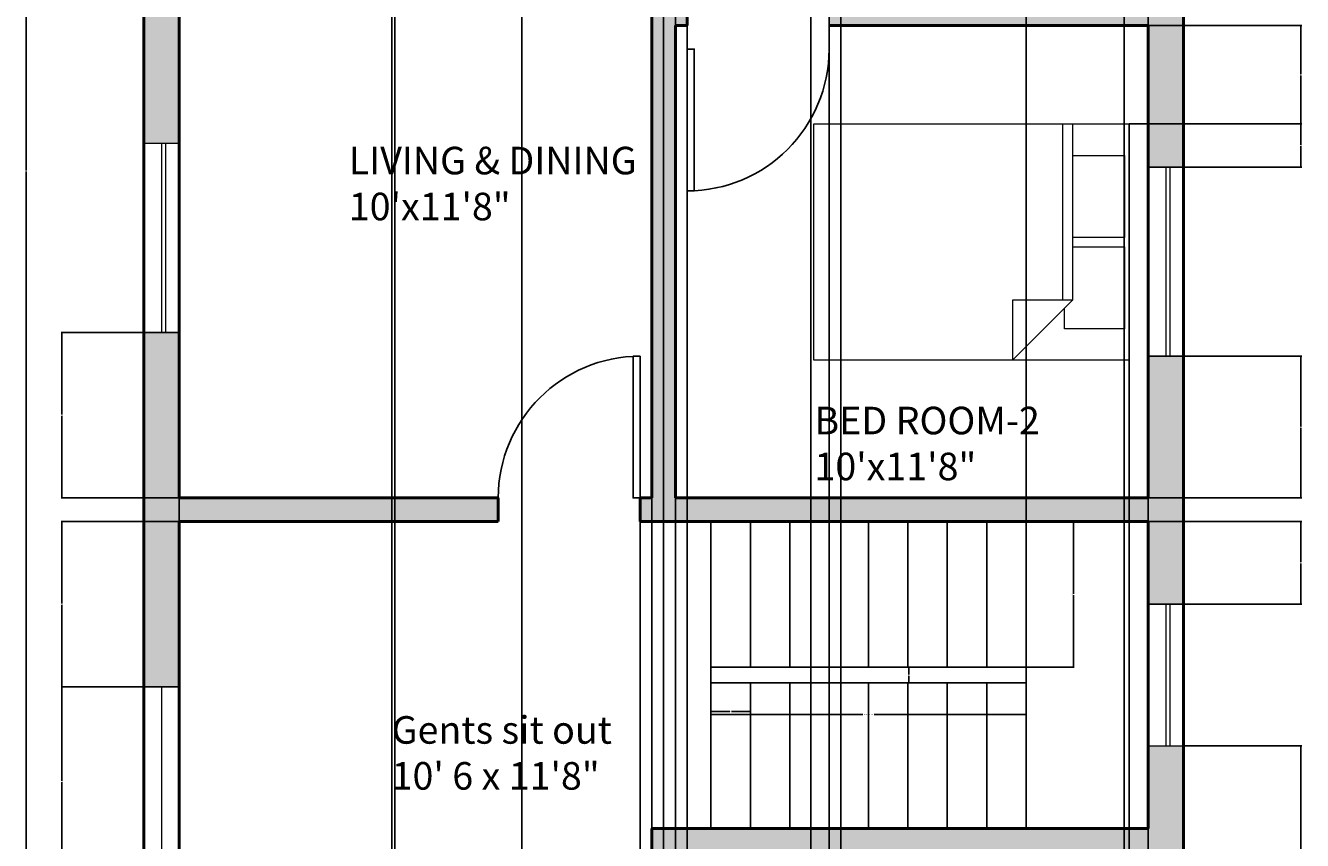
# Model space of a CAD drawing. Units: inches. Extents: x 1489 to 1813, y 1703 to 2293.
# Tile 2 of 4: x 1489 to 1813, y 1843 to 2050. Entities that reach past the tile are written whole.
import ezdxf

# ---------------------------------------------------------------- set-up
doc = ezdxf.new("R2010")
doc.units = ezdxf.units.IN
doc.header["$LTSCALE"] = 0.4
doc.linetypes.add('HIDDEN', pattern=[9.525, 6.35, -3.175])
for name, color, linetype, lineweight in [('A-ANNO-DIMS', 2, 'Continuous', 18), ('A-AREA-IDEN', 7, 'Continuous', 18), ('A-DOOR', 4, 'Continuous', 25), ('A-FLOR-STRS', 7, 'Continuous', 25), ('A-FURN', 8, 'Continuous', 18), ('A-GLAZ', 4, 'Continuous', 18), ('A-WALL', 7, 'Continuous', 50)]:
    doc.layers.add(name, color=color, linetype=linetype, lineweight=lineweight)
doc.layers.add('A-WALL-PATT', color=18, linetype='HIDDEN', lineweight=13, true_color=0x000000)
doc.styles.get("Standard").update_dxf_attribs({"font": 'arial.ttf'})
doc.dimstyles.get("Standard").update_dxf_attribs({"dimtxt": 0.18, "dimasz": 0.18, "dimexe": 0.18, "dimexo": 0.0625, "dimgap": 0.09, "dimtad": 0, "dimtih": 1, "dimtoh": 1, "dimdec": 4, "dimzin": 0, "dimdsep": 46, "dimtxsty": 'Standard', "dimcen": 0.09, "dimadec": 0, "dimazin": 0, "dimtfac": 1, "dimtdec": 4, "dimtofl": 0, "dimtmove": 0, "dimatfit": 3, "dimfxl": 1, "dimtolj": 1, "dimtzin": 0, "dimarcsym": 0})

# ---------------------------------------------------------------- blocks, each defined once
blk = doc.blocks.new('*U5')
for p, q in [((-36, 0), (-36, -6)), ((0, 0), (0, -6))]:
    blk.add_line(p, q)
blk.add_lwpolyline([(0, 0), (0, 36), (-1.75, 36), (-1.75, 0)], close=True)
blk.add_arc((0, 0), 36, 90, 180)
blk = doc.blocks.new('*U4')
for p, q in [((0, 0), (0, -6)), ((36, 0), (36, -6))]:
    blk.add_line(p, q)
blk.add_lwpolyline([(0, 0), (0, 36), (1.75, 36), (1.75, 0)], close=True)
blk.add_arc((0, 0), 36, 0, 90)
blk = doc.blocks.new('Bed - Queen')
for p, q in [((0, -80.00003), (0, 0)), ((0, 0), (59.99999, 0)), ((59.99999, 0), (59.99999, -80.00003)), ((7.99999, -1.2), (28.79998, -1.2)), ((7.99999, -14.4), (7.99999, -1.2)), ((28.79998, -1.2), (28.79998, -14.4)), ((31.19999, -1.2), (51.99999, -1.2)), ((31.19999, -14.4), (31.19999, -1.2)), ((51.99999, -1.2), (51.99999, -16.4)), ((0, -14.4), (44.8, -14.4)), ((59.99999, -29.6), (44.8, -14.4)), ((44.8, -14.4), (44.8, -29.6)), ((44.8, -16.8), (0, -16.8)), ((51.99999, -16.4), (46.79936, -16.4)), ((44.8, -29.6), (59.99999, -29.6)), ((59.99999, -80.00003), (0, -80.00003))]:
    blk.add_line(p, q)
blk = doc.blocks.new('WIN-48IN')
for p, q in [((9, 48), (0, 48)), ((4.5, 48), (4.5, 0)), ((5.5, 48), (5.5, 0)), ((9, 0), (0, 0))]:
    blk.add_line(p, q)
blk = doc.blocks.new('WIN-36IN')
for p, q in [((0, 36), (9, 36)), ((4.5, 36), (4.5, 0)), ((5.5, 36), (5.5, 0)), ((0, 0), (9, 0))]:
    blk.add_line(p, q)
blk = doc.blocks.new('STAIR-FLIGHT-8T')
for p, q in [((10, 37), (10, 0)), ((20, 37), (20, 0)), ((30, 37), (30, 0)), ((40, 37), (40, 0)), ((50, 37), (50, 0)), ((60, 37), (60, 0)), ((70, 37), (70, 0)), ((80, 37), (80, 0)), ((80, 0), (0, 0))]:
    blk.add_line(p, q)
blk = doc.blocks.new('*D20')
at = {"layer": 'A-ANNO-DIMS', "color": 0, "lineweight": -2, "ltscale": 0.4, "transparency": 16777216}
for p, q in [((1663, 1887.11), (1663, 1874.99)), ((1743, 1887.11), (1743, 1874.99)), ((1663.18, 1875.17), (1701.59, 1875.17)), ((1742.82, 1875.17), (1704.42, 1875.17))]:
    blk.add_line(p, q, dxfattribs=at)
at = {"layer": 'A-ANNO-DIMS', "color": 0, "ltscale": 0.4, "transparency": 16777216}
for points in [[(1663.18, 1875.2), (1663.18, 1875.14), (1663, 1875.17)], [(1742.82, 1875.2), (1742.82, 1875.14), (1743, 1875.17)]]:
    blk.add_solid(points, dxfattribs=at)
at = {"layer": 'Defpoints', "color": 0, "ltscale": 0.4, "transparency": 16777216}
for p in [(1663, 1887.17), (1743, 1887.17), (1743, 1875.17)]:
    blk.add_point(p, dxfattribs=at)
at = {"layer": 'A-ANNO-DIMS', "color": 0, "ltscale": 0.4, "transparency": 16777216, "insert": (1703, 1875.17), "char_height": 0.18, "attachment_point": 5}
blk.add_mtext('\\A1;STAIR FLIGHT 80 TYP.', dxfattribs=at)
blk = doc.blocks.new('*D21')
at = {"layer": 'A-ANNO-DIMS', "color": 0, "lineweight": -2, "ltscale": 0.4, "transparency": 16777216}
for p, q in [((1743.06, 1924.17), (1755.18, 1924.17)), ((1755, 1923.99), (1755, 1905.85)), ((1755, 1887.35), (1755, 1905.49)), ((1743.06, 1887.17), (1755.18, 1887.17))]:
    blk.add_line(p, q, dxfattribs=at)
at = {"layer": 'A-ANNO-DIMS', "color": 0, "ltscale": 0.4, "transparency": 16777216}
for points in [[(1754.97, 1923.99), (1755.03, 1923.99), (1755, 1924.17)], [(1754.97, 1887.35), (1755.03, 1887.35), (1755, 1887.17)]]:
    blk.add_solid(points, dxfattribs=at)
at = {"layer": 'Defpoints', "color": 0, "ltscale": 0.4, "transparency": 16777216}
for p in [(1743, 1924.17), (1755, 1924.17), (1743, 1887.17)]:
    blk.add_point(p, dxfattribs=at)
at = {"layer": 'A-ANNO-DIMS', "color": 0, "ltscale": 0.4, "transparency": 16777216, "insert": (1755, 1905.67), "char_height": 0.18, "attachment_point": 5}
blk.add_mtext('\\A1;37 TYP.', dxfattribs=at)
blk = doc.blocks.new('*D29')
at = {"layer": 'A-ANNO-DIMS', "color": 0, "lineweight": -2, "ltscale": 0.4, "transparency": 16777216}
for p, q in [((1518.92, 2263.17), (1489, 2263.17)), ((1489.18, 2262.99), (1489.18, 2013.35)), ((1489.18, 1763.35), (1489.18, 2012.99)), ((1602.92, 1763.17), (1489, 1763.17))]:
    blk.add_line(p, q, dxfattribs=at)
at = {"layer": 'A-ANNO-DIMS', "color": 0, "ltscale": 0.4, "transparency": 16777216}
for points in [[(1489.15, 2262.99), (1489.21, 2262.99), (1489.18, 2263.17)], [(1489.15, 1763.35), (1489.21, 1763.35), (1489.18, 1763.17)]]:
    blk.add_solid(points, dxfattribs=at)
at = {"layer": 'Defpoints', "color": 0, "ltscale": 0.4, "transparency": 16777216}
for p in [(1489.18, 2263.17), (1518.98, 2263.17), (1602.98, 1763.17)]:
    blk.add_point(p, dxfattribs=at)
at = {"layer": 'A-ANNO-DIMS', "color": 0, "ltscale": 0.4, "transparency": 16777216, "insert": (1489.18, 2013.17), "char_height": 0.18, "attachment_point": 5}
blk.add_mtext('\\A1;500', dxfattribs=at)
blk = doc.blocks.new('*D33')
at = {"layer": 'A-ANNO-DIMS', "color": 0, "lineweight": -2, "ltscale": 0.4, "transparency": 16777216}
for p, q in [((1614.98, 1783.23), (1614.98, 2293.15)), ((1615.16, 2292.97), (1632.77, 2292.97)), ((1650.8, 2292.97), (1633.2, 2292.97)), ((1650.98, 1783.23), (1650.98, 2293.15))]:
    blk.add_line(p, q, dxfattribs=at)
at = {"layer": 'A-ANNO-DIMS', "color": 0, "ltscale": 0.4, "transparency": 16777216}
for points in [[(1615.16, 2293), (1615.16, 2292.94), (1614.98, 2292.97)], [(1650.8, 2293), (1650.8, 2292.94), (1650.98, 2292.97)]]:
    blk.add_solid(points, dxfattribs=at)
at = {"layer": 'Defpoints', "color": 0, "ltscale": 0.4, "transparency": 16777216}
for p in [(1650.98, 2292.97), (1614.98, 1783.17), (1650.98, 1783.17)]:
    blk.add_point(p, dxfattribs=at)
at = {"layer": 'A-ANNO-DIMS', "color": 0, "ltscale": 0.4, "transparency": 16777216, "insert": (1632.98, 2292.97), "char_height": 0.18, "attachment_point": 5}
blk.add_mtext('\\A1;36', dxfattribs=at)
blk = doc.blocks.new('*D34')
at = {"layer": 'A-ANNO-DIMS', "color": 0, "lineweight": -2, "ltscale": 0.4, "transparency": 16777216}
for p, q in [((1783.05, 1867.17), (1812.96, 1867.17)), ((1812.78, 1866.99), (1812.78, 1825.35)), ((1812.78, 1783.35), (1812.78, 1824.99)), ((1783.05, 1783.17), (1812.96, 1783.17))]:
    blk.add_line(p, q, dxfattribs=at)
at = {"layer": 'A-ANNO-DIMS', "color": 0, "ltscale": 0.4, "transparency": 16777216}
for points in [[(1812.75, 1866.99), (1812.81, 1866.99), (1812.78, 1867.17)], [(1812.75, 1783.35), (1812.81, 1783.35), (1812.78, 1783.17)]]:
    blk.add_solid(points, dxfattribs=at)
at = {"layer": 'Defpoints', "color": 0, "ltscale": 0.4, "transparency": 16777216}
for p in [(1782.98, 1867.17), (1812.78, 1867.17), (1782.98, 1783.17)]:
    blk.add_point(p, dxfattribs=at)
at = {"layer": 'A-ANNO-DIMS', "color": 0, "ltscale": 0.4, "transparency": 16777216, "insert": (1812.78, 1825.17), "char_height": 0.18, "attachment_point": 5}
blk.add_mtext('\\A1;84', dxfattribs=at)
blk = doc.blocks.new('*D35')
at = {"layer": 'A-ANNO-DIMS', "color": 0, "lineweight": -2, "ltscale": 0.4, "transparency": 16777216}
for p, q in [((1774.05, 1924.17), (1812.96, 1924.17)), ((1812.78, 1923.99), (1812.78, 1913.85)), ((1812.78, 1903.35), (1812.78, 1913.49)), ((1774.05, 1903.17), (1812.96, 1903.17))]:
    blk.add_line(p, q, dxfattribs=at)
at = {"layer": 'A-ANNO-DIMS', "color": 0, "ltscale": 0.4, "transparency": 16777216}
for points in [[(1812.75, 1923.99), (1812.81, 1923.99), (1812.78, 1924.17)], [(1812.75, 1903.35), (1812.81, 1903.35), (1812.78, 1903.17)]]:
    blk.add_solid(points, dxfattribs=at)
at = {"layer": 'Defpoints', "color": 0, "ltscale": 0.4, "transparency": 16777216}
for p in [(1773.98, 1924.17), (1812.78, 1924.17), (1773.98, 1903.17)]:
    blk.add_point(p, dxfattribs=at)
at = {"layer": 'A-ANNO-DIMS', "color": 0, "ltscale": 0.4, "transparency": 16777216, "insert": (1812.78, 1913.67), "char_height": 0.18, "attachment_point": 5}
blk.add_mtext('\\A1;21', dxfattribs=at)
blk = doc.blocks.new('*D36')
at = {"layer": 'A-ANNO-DIMS', "color": 0, "lineweight": -2, "ltscale": 0.4, "transparency": 16777216}
for p, q in [((1774.05, 1966.17), (1812.96, 1966.17)), ((1812.78, 1965.99), (1812.78, 1948.35)), ((1812.78, 1930.35), (1812.78, 1947.99)), ((1774.05, 1930.17), (1812.96, 1930.17))]:
    blk.add_line(p, q, dxfattribs=at)
at = {"layer": 'A-ANNO-DIMS', "color": 0, "ltscale": 0.4, "transparency": 16777216}
for points in [[(1812.75, 1965.99), (1812.81, 1965.99), (1812.78, 1966.17)], [(1812.75, 1930.35), (1812.81, 1930.35), (1812.78, 1930.17)]]:
    blk.add_solid(points, dxfattribs=at)
at = {"layer": 'Defpoints', "color": 0, "ltscale": 0.4, "transparency": 16777216}
for p in [(1773.98, 1966.17), (1812.78, 1966.17), (1773.98, 1930.17)]:
    blk.add_point(p, dxfattribs=at)
at = {"layer": 'A-ANNO-DIMS', "color": 0, "ltscale": 0.4, "transparency": 16777216, "insert": (1812.78, 1948.17), "char_height": 0.18, "attachment_point": 5}
blk.add_mtext('\\A1;36', dxfattribs=at)
blk = doc.blocks.new('*D37')
at = {"layer": 'A-ANNO-DIMS', "color": 0, "lineweight": -2, "ltscale": 0.4, "transparency": 16777216}
for p, q in [((1769.2, 2025.17), (1812.96, 2025.17)), ((1812.78, 2024.99), (1812.78, 2019.85)), ((1812.78, 2014.35), (1812.78, 2019.49)), ((1774.05, 2014.17), (1812.96, 2014.17))]:
    blk.add_line(p, q, dxfattribs=at)
at = {"layer": 'A-ANNO-DIMS', "color": 0, "ltscale": 0.4, "transparency": 16777216}
for points in [[(1812.75, 2024.99), (1812.81, 2024.99), (1812.78, 2025.17)], [(1812.75, 2014.35), (1812.81, 2014.35), (1812.78, 2014.17)]]:
    blk.add_solid(points, dxfattribs=at)
at = {"layer": 'Defpoints', "color": 0, "ltscale": 0.4, "transparency": 16777216}
for p in [(1769.14, 2025.17), (1812.78, 2025.17), (1773.98, 2014.17)]:
    blk.add_point(p, dxfattribs=at)
at = {"layer": 'A-ANNO-DIMS', "color": 0, "ltscale": 0.4, "transparency": 16777216, "insert": (1812.78, 2019.67), "char_height": 0.18, "attachment_point": 5}
blk.add_mtext('\\A1;10.999', dxfattribs=at)
blk = doc.blocks.new('*D41')
at = {"layer": 'A-ANNO-DIMS', "color": 0, "lineweight": -2, "ltscale": 0.4, "transparency": 16777216}
for p, q in [((1647.98, 2254.11), (1647.98, 1705.95)), ((1653.98, 2254.11), (1653.98, 1705.95)), ((1648.16, 1706.13), (1650.83, 1706.13)), ((1653.8, 1706.13), (1651.13, 1706.13))]:
    blk.add_line(p, q, dxfattribs=at)
at = {"layer": 'A-ANNO-DIMS', "color": 0, "ltscale": 0.4, "transparency": 16777216}
for points in [[(1648.16, 1706.16), (1648.16, 1706.1), (1647.98, 1706.13)], [(1653.8, 1706.16), (1653.8, 1706.1), (1653.98, 1706.13)]]:
    blk.add_solid(points, dxfattribs=at)
at = {"layer": 'Defpoints', "color": 0, "ltscale": 0.4, "transparency": 16777216}
for p in [(1647.98, 2254.17), (1653.98, 2254.17), (1653.98, 1706.13)]:
    blk.add_point(p, dxfattribs=at)
at = {"layer": 'A-ANNO-DIMS', "color": 0, "ltscale": 0.4, "transparency": 16777216, "insert": (1650.98, 1706.13), "char_height": 0.18, "attachment_point": 5}
blk.add_mtext('\\A1;6', dxfattribs=at)
blk = doc.blocks.new('*D42')
at = {"layer": 'A-ANNO-DIMS', "color": 0, "lineweight": -2, "ltscale": 0.4, "transparency": 16777216}
for p, q in [((1527.92, 1882.17), (1498, 1882.17)), ((1498.18, 1881.99), (1498.18, 1858.35)), ((1498.18, 1834.35), (1498.18, 1857.99)), ((1527.92, 1834.17), (1498, 1834.17))]:
    blk.add_line(p, q, dxfattribs=at)
at = {"layer": 'A-ANNO-DIMS', "color": 0, "ltscale": 0.4, "transparency": 16777216}
for points in [[(1498.15, 1881.99), (1498.21, 1881.99), (1498.18, 1882.17)], [(1498.15, 1834.35), (1498.21, 1834.35), (1498.18, 1834.17)]]:
    blk.add_solid(points, dxfattribs=at)
at = {"layer": 'Defpoints', "color": 0, "ltscale": 0.4, "transparency": 16777216}
for p in [(1498.18, 1882.17), (1527.98, 1882.17), (1527.98, 1834.17)]:
    blk.add_point(p, dxfattribs=at)
at = {"layer": 'A-ANNO-DIMS', "color": 0, "ltscale": 0.4, "transparency": 16777216, "insert": (1498.18, 1858.17), "char_height": 0.18, "attachment_point": 5}
blk.add_mtext('\\A1;48', dxfattribs=at)
blk = doc.blocks.new('*D43')
at = {"layer": 'A-ANNO-DIMS', "color": 0, "lineweight": -2, "ltscale": 0.4, "transparency": 16777216}
for p, q in [((1527.92, 1924.17), (1498, 1924.17)), ((1498.18, 1923.99), (1498.18, 1903.35)), ((1498.18, 1882.35), (1498.18, 1902.99)), ((1527.92, 1882.17), (1498, 1882.17))]:
    blk.add_line(p, q, dxfattribs=at)
at = {"layer": 'A-ANNO-DIMS', "color": 0, "ltscale": 0.4, "transparency": 16777216}
for points in [[(1498.15, 1923.99), (1498.21, 1923.99), (1498.18, 1924.17)], [(1498.15, 1882.35), (1498.21, 1882.35), (1498.18, 1882.17)]]:
    blk.add_solid(points, dxfattribs=at)
at = {"layer": 'Defpoints', "color": 0, "ltscale": 0.4, "transparency": 16777216}
for p in [(1498.18, 1924.17), (1527.98, 1924.17), (1527.98, 1882.17)]:
    blk.add_point(p, dxfattribs=at)
at = {"layer": 'A-ANNO-DIMS', "color": 0, "ltscale": 0.4, "transparency": 16777216, "insert": (1498.18, 1903.17), "char_height": 0.18, "attachment_point": 5}
blk.add_mtext('\\A1;42', dxfattribs=at)
blk = doc.blocks.new('*D44')
at = {"layer": 'A-ANNO-DIMS', "color": 0, "lineweight": -2, "ltscale": 0.4, "transparency": 16777216}
for p, q in [((1527.92, 1972.17), (1498, 1972.17)), ((1498.18, 1971.99), (1498.18, 1951.35)), ((1498.18, 1930.35), (1498.18, 1950.99)), ((1527.92, 1930.17), (1498, 1930.17))]:
    blk.add_line(p, q, dxfattribs=at)
at = {"layer": 'A-ANNO-DIMS', "color": 0, "ltscale": 0.4, "transparency": 16777216}
for points in [[(1498.15, 1971.99), (1498.21, 1971.99), (1498.18, 1972.17)], [(1498.15, 1930.35), (1498.21, 1930.35), (1498.18, 1930.17)]]:
    blk.add_solid(points, dxfattribs=at)
at = {"layer": 'Defpoints', "color": 0, "ltscale": 0.4, "transparency": 16777216}
for p in [(1498.18, 1972.17), (1527.98, 1972.17), (1527.98, 1930.17)]:
    blk.add_point(p, dxfattribs=at)
at = {"layer": 'A-ANNO-DIMS', "color": 0, "ltscale": 0.4, "transparency": 16777216, "insert": (1498.18, 1951.17), "char_height": 0.18, "attachment_point": 5}
blk.add_mtext('\\A1;42', dxfattribs=at)
blk = doc.blocks.new('*D49')
at = {"layer": 'A-ANNO-DIMS', "color": 0, "lineweight": -2, "ltscale": 0.4, "transparency": 16777216}
for p, q in [((1743, 1846.23), (1743, 2293.15)), ((1743.18, 2292.97), (1758.03, 2292.97)), ((1773.8, 2292.97), (1758.96, 2292.97)), ((1773.98, 1846.23), (1773.98, 2293.15))]:
    blk.add_line(p, q, dxfattribs=at)
at = {"layer": 'A-ANNO-DIMS', "color": 0, "ltscale": 0.4, "transparency": 16777216}
for points in [[(1743.18, 2293), (1743.18, 2292.94), (1743, 2292.97)], [(1773.8, 2293), (1773.8, 2292.94), (1773.98, 2292.97)]]:
    blk.add_solid(points, dxfattribs=at)
at = {"layer": 'Defpoints', "color": 0, "ltscale": 0.4, "transparency": 16777216}
for p in [(1773.98, 2292.97), (1743, 1846.17), (1773.98, 1846.17)]:
    blk.add_point(p, dxfattribs=at)
at = {"layer": 'A-ANNO-DIMS', "color": 0, "ltscale": 0.4, "transparency": 16777216, "insert": (1758.49, 2292.97), "char_height": 0.18, "attachment_point": 5}
blk.add_mtext('\\A1;30.983', dxfattribs=at)
blk = doc.blocks.new('*D50')
at = {"layer": 'A-ANNO-DIMS', "color": 0, "lineweight": -2, "ltscale": 0.4, "transparency": 16777216}
for p, q in [((1742.93793, 1887.170878), (1713.02043, 1887.170878)), ((1713.20043, 1886.990878), (1713.20043, 1885.350878)), ((1713.20043, 1883.350878), (1713.20043, 1884.990878)), ((1742.93793, 1883.170878), (1713.02043, 1883.170878))]:
    blk.add_line(p, q, dxfattribs=at)
at = {"layer": 'A-ANNO-DIMS', "color": 0, "ltscale": 0.4, "transparency": 16777216}
for points in [[(1713.17043, 1886.990878), (1713.23043, 1886.990878), (1713.20043, 1887.170878)], [(1713.17043, 1883.350878), (1713.23043, 1883.350878), (1713.20043, 1883.170878)]]:
    blk.add_solid(points, dxfattribs=at)
at = {"layer": 'Defpoints', "color": 0, "ltscale": 0.4, "transparency": 16777216}
for p in [(1713.20043, 1887.170878), (1743.00043, 1887.170878), (1743.00043, 1883.170878)]:
    blk.add_point(p, dxfattribs=at)
at = {"layer": 'A-ANNO-DIMS', "color": 0, "ltscale": 0.4, "transparency": 16777216, "insert": (1713.20043, 1885.170878), "char_height": 0.18, "attachment_point": 5}
blk.add_mtext('\\A1;4', dxfattribs=at)
blk = doc.blocks.new('*D52')
at = {"layer": 'A-ANNO-DIMS', "color": 0, "lineweight": -2, "ltscale": 0.4, "transparency": 16777216}
for p, q in [((1527.98, 2254.11), (1527.98, 1705.95)), ((1582.71, 2254.11), (1582.71, 1705.95)), ((1528.16, 1706.13), (1554.95, 1706.13)), ((1582.53, 1706.13), (1555.74, 1706.13))]:
    blk.add_line(p, q, dxfattribs=at)
at = {"layer": 'A-ANNO-DIMS', "color": 0, "ltscale": 0.4, "transparency": 16777216}
for points in [[(1528.16, 1706.16), (1528.16, 1706.1), (1527.98, 1706.13)], [(1582.53, 1706.16), (1582.53, 1706.1), (1582.71, 1706.13)]]:
    blk.add_solid(points, dxfattribs=at)
at = {"layer": 'Defpoints', "color": 0, "ltscale": 0.4, "transparency": 16777216}
for p in [(1527.98, 2254.17), (1582.71, 2254.17), (1582.71, 1706.13)]:
    blk.add_point(p, dxfattribs=at)
at = {"layer": 'A-ANNO-DIMS', "color": 0, "ltscale": 0.4, "transparency": 16777216, "insert": (1555.35, 1706.13), "char_height": 0.18, "attachment_point": 5}
blk.add_mtext('\\A1;54.73', dxfattribs=at)
blk = doc.blocks.new('*D53')
at = {"layer": 'A-ANNO-DIMS', "color": 0, "lineweight": -2, "ltscale": 0.4, "transparency": 16777216}
for p, q in [((1656.98, 2122.11), (1656.98, 1705.95)), ((1692.98, 2122.11), (1692.98, 1705.95)), ((1657.16, 1706.13), (1674.77, 1706.13)), ((1692.8, 1706.13), (1675.2, 1706.13))]:
    blk.add_line(p, q, dxfattribs=at)
at = {"layer": 'A-ANNO-DIMS', "color": 0, "ltscale": 0.4, "transparency": 16777216}
for points in [[(1657.16, 1706.16), (1657.16, 1706.1), (1656.98, 1706.13)], [(1692.8, 1706.16), (1692.8, 1706.1), (1692.98, 1706.13)]]:
    blk.add_solid(points, dxfattribs=at)
at = {"layer": 'Defpoints', "color": 0, "ltscale": 0.4, "transparency": 16777216}
for p in [(1656.98, 2122.17), (1692.98, 2122.17), (1692.98, 1706.13)]:
    blk.add_point(p, dxfattribs=at)
at = {"layer": 'A-ANNO-DIMS', "color": 0, "ltscale": 0.4, "transparency": 16777216, "insert": (1674.98, 1706.13), "char_height": 0.18, "attachment_point": 5}
blk.add_mtext('\\A1;36', dxfattribs=at)
blk = doc.blocks.new('*D55')
at = {"layer": 'A-ANNO-DIMS', "color": 0, "lineweight": -2, "ltscale": 0.4, "transparency": 16777216}
for p, q in [((1663, 1846.23), (1663, 1876.15)), ((1663.18, 1875.97), (1667.79, 1875.97)), ((1672.82, 1875.97), (1668.21, 1875.97)), ((1673, 1846.23), (1673, 1876.15))]:
    blk.add_line(p, q, dxfattribs=at)
at = {"layer": 'A-ANNO-DIMS', "color": 0, "ltscale": 0.4, "transparency": 16777216}
for points in [[(1663.18, 1876), (1663.18, 1875.94), (1663, 1875.97)], [(1672.82, 1876), (1672.82, 1875.94), (1673, 1875.97)]]:
    blk.add_solid(points, dxfattribs=at)
at = {"layer": 'Defpoints', "color": 0, "ltscale": 0.4, "transparency": 16777216}
for p in [(1673, 1875.97), (1663, 1846.17), (1673, 1846.17)]:
    blk.add_point(p, dxfattribs=at)
at = {"layer": 'A-ANNO-DIMS', "color": 0, "ltscale": 0.4, "transparency": 16777216, "insert": (1668, 1875.97), "char_height": 0.18, "attachment_point": 5}
blk.add_mtext('\\A1;10', dxfattribs=at)
blk = doc.blocks.new('*D57')
at = {"layer": 'A-ANNO-DIMS', "color": 0, "lineweight": -2, "ltscale": 0.4, "transparency": 16777216}
for p, q in [((1644.98, 1930.11), (1644.98, 1705.95)), ((1647.98, 1930.11), (1647.98, 1705.95)), ((1645.16, 1706.13), (1646.33, 1706.13)), ((1647.8, 1706.13), (1646.63, 1706.13))]:
    blk.add_line(p, q, dxfattribs=at)
at = {"layer": 'A-ANNO-DIMS', "color": 0, "ltscale": 0.4, "transparency": 16777216}
for points in [[(1645.16, 1706.16), (1645.16, 1706.1), (1644.98, 1706.13)], [(1647.8, 1706.16), (1647.8, 1706.1), (1647.98, 1706.13)]]:
    blk.add_solid(points, dxfattribs=at)
at = {"layer": 'Defpoints', "color": 0, "ltscale": 0.4, "transparency": 16777216}
for p in [(1644.98, 1930.17), (1647.98, 1930.17), (1647.98, 1706.13)]:
    blk.add_point(p, dxfattribs=at)
at = {"layer": 'A-ANNO-DIMS', "color": 0, "ltscale": 0.4, "transparency": 16777216, "insert": (1646.48, 1706.13), "char_height": 0.18, "attachment_point": 5}
blk.add_mtext('\\A1;3', dxfattribs=at)
blk = doc.blocks.new('*D59')
at = {"layer": 'A-ANNO-DIMS', "color": 0, "lineweight": -2, "ltscale": 0.4, "transparency": 16777216}
for p, q in [((1653.98, 2254.11), (1653.98, 1705.95)), ((1688.31, 2248.43), (1688.31, 1705.95)), ((1654.16, 1706.13), (1670.75, 1706.13)), ((1688.13, 1706.13), (1671.54, 1706.13))]:
    blk.add_line(p, q, dxfattribs=at)
at = {"layer": 'A-ANNO-DIMS', "color": 0, "ltscale": 0.4, "transparency": 16777216}
for points in [[(1654.16, 1706.16), (1654.16, 1706.1), (1653.98, 1706.13)], [(1688.13, 1706.16), (1688.13, 1706.1), (1688.31, 1706.13)]]:
    blk.add_solid(points, dxfattribs=at)
at = {"layer": 'Defpoints', "color": 0, "ltscale": 0.4, "transparency": 16777216}
for p in [(1653.98, 2254.17), (1688.31, 2248.49), (1688.31, 1706.13)]:
    blk.add_point(p, dxfattribs=at)
at = {"layer": 'A-ANNO-DIMS', "color": 0, "ltscale": 0.4, "transparency": 16777216, "insert": (1671.14, 1706.13), "char_height": 0.18, "attachment_point": 5}
blk.add_mtext('\\A1;34.32', dxfattribs=at)
blk = doc.blocks.new('*D61')
at = {"layer": 'A-ANNO-DIMS', "color": 0, "lineweight": -2, "ltscale": 0.4, "transparency": 16777216}
for p, q in [((1773.98, 2050.11), (1773.98, 1705.95)), ((1769.14, 2025.11), (1769.14, 1705.95)), ((1769.32, 1706.13), (1771.17, 1706.13)), ((1773.8, 1706.13), (1771.96, 1706.13))]:
    blk.add_line(p, q, dxfattribs=at)
at = {"layer": 'A-ANNO-DIMS', "color": 0, "ltscale": 0.4, "transparency": 16777216}
for points in [[(1769.32, 1706.16), (1769.32, 1706.1), (1769.14, 1706.13)], [(1773.8, 1706.16), (1773.8, 1706.1), (1773.98, 1706.13)]]:
    blk.add_solid(points, dxfattribs=at)
at = {"layer": 'Defpoints', "color": 0, "ltscale": 0.4, "transparency": 16777216}
for p in [(1773.98, 2050.17), (1769.14, 2025.17), (1773.98, 1706.13)]:
    blk.add_point(p, dxfattribs=at)
at = {"layer": 'A-ANNO-DIMS', "color": 0, "ltscale": 0.4, "transparency": 16777216, "insert": (1771.56, 1706.13), "char_height": 0.18, "attachment_point": 5}
blk.add_mtext('\\A1;4.844', dxfattribs=at)
blk = doc.blocks.new('*D62')
at = {"layer": 'A-ANNO-DIMS', "color": 0, "lineweight": -2, "ltscale": 0.4, "transparency": 16777216}
for p, q in [((1774.05, 2050.17), (1812.96, 2050.17)), ((1812.78, 2049.99), (1812.78, 2037.85)), ((1812.78, 2025.35), (1812.78, 2037.49)), ((1769.2, 2025.17), (1812.96, 2025.17))]:
    blk.add_line(p, q, dxfattribs=at)
at = {"layer": 'A-ANNO-DIMS', "color": 0, "ltscale": 0.4, "transparency": 16777216}
for points in [[(1812.75, 2049.99), (1812.81, 2049.99), (1812.78, 2050.17)], [(1812.75, 2025.35), (1812.81, 2025.35), (1812.78, 2025.17)]]:
    blk.add_solid(points, dxfattribs=at)
at = {"layer": 'Defpoints', "color": 0, "ltscale": 0.4, "transparency": 16777216}
for p in [(1773.98, 2050.17), (1812.78, 2050.17), (1769.14, 2025.17)]:
    blk.add_point(p, dxfattribs=at)
at = {"layer": 'A-ANNO-DIMS', "color": 0, "ltscale": 0.4, "transparency": 16777216, "insert": (1812.78, 2037.67), "char_height": 0.18, "attachment_point": 5}
blk.add_mtext('\\A1;25', dxfattribs=at)
blk = doc.blocks.new('*D63')
at = {"layer": 'A-ANNO-DIMS', "color": 0, "lineweight": -2, "ltscale": 0.4, "transparency": 16777216}
for p, q in [((1581.98, 2062.11), (1581.98, 1705.95)), ((1695.98, 2056.11), (1695.98, 1705.95)), ((1582.16, 1706.13), (1638.7, 1706.13)), ((1695.8, 1706.13), (1639.26, 1706.13))]:
    blk.add_line(p, q, dxfattribs=at)
at = {"layer": 'A-ANNO-DIMS', "color": 0, "ltscale": 0.4, "transparency": 16777216}
for points in [[(1582.16, 1706.16), (1582.16, 1706.1), (1581.98, 1706.13)], [(1695.8, 1706.16), (1695.8, 1706.1), (1695.98, 1706.13)]]:
    blk.add_solid(points, dxfattribs=at)
at = {"layer": 'Defpoints', "color": 0, "ltscale": 0.4, "transparency": 16777216}
for p in [(1581.98, 2062.17), (1695.98, 2056.17), (1695.98, 1706.13)]:
    blk.add_point(p, dxfattribs=at)
at = {"layer": 'A-ANNO-DIMS', "color": 0, "ltscale": 0.4, "transparency": 16777216, "insert": (1638.98, 1706.13), "char_height": 0.18, "attachment_point": 5}
blk.add_mtext('\\A1;114', dxfattribs=at)
blk = doc.blocks.new('*D64')
at = {"layer": 'A-ANNO-DIMS', "color": 0, "lineweight": -2, "ltscale": 0.4, "transparency": 16777216}
for p, q in [((1767.89, 2061.85), (1767.89, 1705.95)), ((1773.98, 2056.11), (1773.98, 1705.95)), ((1768.07, 1706.13), (1770.56, 1706.13)), ((1773.8, 1706.13), (1771.31, 1706.13))]:
    blk.add_line(p, q, dxfattribs=at)
at = {"layer": 'A-ANNO-DIMS', "color": 0, "ltscale": 0.4, "transparency": 16777216}
for points in [[(1768.07, 1706.16), (1768.07, 1706.1), (1767.89, 1706.13)], [(1773.8, 1706.16), (1773.8, 1706.1), (1773.98, 1706.13)]]:
    blk.add_solid(points, dxfattribs=at)
at = {"layer": 'Defpoints', "color": 0, "ltscale": 0.4, "transparency": 16777216}
for p in [(1767.89, 2061.91), (1773.98, 2056.17), (1773.98, 1706.13)]:
    blk.add_point(p, dxfattribs=at)
at = {"layer": 'A-ANNO-DIMS', "color": 0, "ltscale": 0.4, "transparency": 16777216, "insert": (1770.94, 1706.13), "char_height": 0.18, "attachment_point": 5}
blk.add_mtext('\\A1;6.091', dxfattribs=at)

msp = doc.modelspace()

# ---------------------------------------------------------------- hatches: boundary and pattern name
at = {"layer": 'A-WALL-PATT', "ltscale": 0.4}
h = msp.add_hatch(dxfattribs=at)
h.set_pattern_fill('HONEY', color=256, scale=0.1)
h.paths.add_polyline_path([(1782.9839, 2263.1709), (1645.9839, 2263.1709), (1645.9839, 2254.1709), (1647.9839, 2254.1709), (1647.9839, 2116.1709), (1653.9839, 2116.1709), (1656.9839, 2116.1709), (1656.9839, 2122.1709), (1653.9839, 2122.1709), (1653.9839, 2254.1709), (1773.9839, 2254.1709), (1773.9839, 2212.1709), (1782.9839, 2212.1709)])
h.paths.add_polyline_path([(1782.9839, 2164.1709), (1773.9839, 2164.1709), (1773.9839, 2122.1709), (1695.9839, 2122.1709), (1692.9839, 2122.1709), (1692.9839, 2116.1709), (1695.9839, 2116.1709), (1695.9839, 2113.1709), (1701.9839, 2113.1709), (1701.9839, 2116.1709), (1773.9839, 2116.1709), (1773.9839, 2104.1709), (1782.9839, 2104.1709)])
h.paths.add_polyline_path([(1782.9839, 2068.1709), (1773.9839, 2068.1709), (1773.9839, 2056.1709), (1701.9839, 2056.1709), (1701.9839, 2083.1709), (1695.9839, 2083.1709), (1695.9839, 2056.1709), (1692.9839, 2056.1709), (1692.9839, 2050.1709), (1695.9839, 2050.1709), (1773.9839, 2050.1709), (1773.9839, 2014.1709), (1782.9839, 2014.1709)])
h = msp.add_hatch(dxfattribs=at)
h.set_pattern_fill('HONEY', color=256, scale=0.1)
h.paths.add_polyline_path([(1527.9839, 2128.1709), (1575.9839, 2128.1709), (1575.9839, 2125.1709), (1581.9839, 2125.1709), (1581.9839, 2134.1709), (1527.9839, 2134.1709), (1527.9839, 2170.1709), (1518.9839, 2170.1709), (1518.9839, 2020.1709), (1527.9839, 2020.1709), (1527.9839, 2062.1709), (1581.9839, 2062.1709), (1581.9839, 2095.1709), (1575.9839, 2095.1709), (1575.9839, 2068.1709), (1527.9839, 2068.1709)])
h.paths.add_polyline_path([(1527.9839, 1924.1709), (1608.9839, 1924.1709), (1608.9839, 1930.1709), (1527.9839, 1930.1709), (1527.9839, 1972.1709), (1518.9839, 1972.1709), (1518.9839, 1882.1709), (1527.9839, 1882.1709)])
h.paths.add_polyline_path([(1527.9839, 1834.1709), (1518.9839, 1834.1709), (1518.9839, 1783.1709), (1614.9839, 1783.1709), (1614.9839, 1789.1709), (1614.9839, 1792.1709), (1527.9839, 1792.1709)])
h.paths.add_polyline_path([(1782.9839, 1867.1709), (1773.9839, 1867.1709), (1773.9839, 1846.1709), (1647.9839, 1846.1709), (1647.9839, 1840.1709), (1773.9839, 1840.1709), (1773.9839, 1792.1709), (1650.9839, 1792.1709), (1650.9839, 1783.1709), (1782.9839, 1783.1709)])
h.paths.add_polyline_path([(1540.5005, 2064.0337), (1577.6874, 2064.0337), (1577.6874, 2090.1253), (1540.5005, 2090.1253)], flags=24)
h = msp.add_hatch(dxfattribs=at)
h.set_pattern_fill('HONEY', color=256, scale=0.1)
h.paths.add_polyline_path([(1653.9839, 2050.1709), (1656.9839, 2050.1709), (1656.9839, 2056.1709), (1653.9839, 2056.1709), (1647.9839, 2056.1709), (1647.9839, 1930.1709), (1644.9839, 1930.1709), (1644.9839, 1924.1709), (1773.9839, 1924.1709), (1773.9839, 1903.1709), (1782.9839, 1903.1709), (1782.9839, 1966.1709), (1773.9839, 1966.1709), (1773.9839, 1930.1709), (1653.9839, 1930.1709)])

# ---------------------------------------------------------------- linework, layer by layer
at = {"layer": 'A-FLOR-STRS'}
msp.add_line((1663.0004, 1924.1709), (1663.0004, 1846.1709), dxfattribs=at)
at = {"layer": 'A-GLAZ'}
for p, q in [((1527.9839, 1882.1709), (1518.9839, 1882.1709)), ((1523.4839, 1882.1709), (1523.4839, 1834.1709))]:
    msp.add_line(p, q, dxfattribs=at)
at = {"layer": 'A-WALL'}
for p, q in [((1518.9839, 2263.1709), (1518.9839, 1783.1709)), ((1782.9839, 1783.1709), (1782.9839, 2263.1709)), ((1527.9839, 2062.1709), (1527.9839, 1930.1709)), ((1647.9839, 2056.1709), (1647.9839, 1930.1709)), ((1656.9839, 2050.1709), (1656.9839, 2056.1709)), ((1653.9839, 1930.1709), (1653.9839, 2050.1709)), ((1653.9839, 2050.1709), (1653.9839, 1930.1709)), ((1656.9839, 2050.1709), (1653.9839, 2050.1709)), ((1695.9839, 2050.1709), (1692.9839, 2050.1709)), ((1773.9839, 2050.1709), (1695.9839, 2050.1709)), ((1773.9839, 1930.1709), (1773.9839, 2050.1709)), ((1527.9839, 1930.1709), (1608.9839, 1930.1709)), ((1608.9839, 1930.1709), (1608.9839, 1924.1709)), ((1644.9839, 1930.1709), (1644.9839, 1924.1709)), ((1644.9839, 1930.1709), (1647.9839, 1930.1709)), ((1653.9839, 1930.1709), (1773.9839, 1930.1709)), ((1527.9839, 1924.1709), (1608.9839, 1924.1709)), ((1527.9839, 1924.1709), (1527.9839, 1792.1709)), ((1644.9839, 1924.1709), (1773.9839, 1924.1709)), ((1773.9839, 1846.1709), (1773.9839, 1924.1709)), ((1647.9839, 1846.1709), (1773.9839, 1846.1709)), ((1647.9839, 1846.1709), (1647.9839, 1840.1709))]:
    msp.add_line(p, q, dxfattribs=at)

# ---------------------------------------------------------------- block references
at = {"layer": 'A-DOOR', "rotation": 180}
msp.add_blockref('*U5', (1656.9839, 2044.1709), dxfattribs=at)
at = {"layer": 'A-DOOR', "xscale": -1}
msp.add_blockref('*U4', (1644.9839, 1930.1709), dxfattribs=at)
at = {"layer": 'A-FLOR-STRS'}
msp.add_blockref('STAIR-FLIGHT-8T', (1663, 1887.171), dxfattribs=at)
at = {"layer": 'A-FLOR-STRS', "extrusion": (0, 0, -1), "zscale": -1, "rotation": 180}
msp.add_blockref('STAIR-FLIGHT-8T', (-1663, 1883.1708), dxfattribs=at)
at = {"layer": 'A-FURN', "rotation": 270}
msp.add_blockref('Bed - Queen', (1769.1403, 2025.1698), dxfattribs=at)
at = {"layer": 'A-GLAZ'}
for name, p in [('WIN-48IN', (1518.984, 1972.171)), ('WIN-48IN', (1773.984, 1966.171)), ('WIN-36IN', (1773.984, 1867.171))]:
    msp.add_blockref(name, p, dxfattribs=at)

# ---------------------------------------------------------------- texts
at = {"layer": 'A-AREA-IDEN', "char_height": 7, "attachment_point": 1}
for s, width, insert in [('LIVING & DINING\\P10\'x11\'8"', 76.937557, (1571.0463, 2019.3685)), ('BED ROOM-2\\P10\'x11\'8"', 72.76642, (1689.2651, 1953.3358)), ('Gents sit out\\P10\' 6 x 11\'8"', 62.358351, (1581.925, 1874.7488))]:
    msp.add_mtext_dynamic_manual_height_columns(s, width=width, gutter_width=12.5, heights=[0], dxfattribs=dict(at, insert=insert))

# ---------------------------------------------------------------- dimensions: what is measured, and where the dimension line sits
at = {"layer": 'A-ANNO-DIMS', "ltscale": 0.4}
for base, p1, p2, override, picture, middle in [((1650.9839, 2292.9709), (1614.9839, 1783.1709), (1650.9839, 1783.1709), {"dimdec": 0, "dimlfac": 1, "dimrnd": 0, "dimzin": 0, "dimdsep": 46, "dimlunit": 2}, '*D33', (1632.9839, 2292.9709)), ((1773.98388, 2292.97088), (1743.00043, 1846.17088), (1773.98388, 1846.17088), {"dimdec": 3, "dimlfac": 1, "dimrnd": 0, "dimzin": 0, "dimdsep": 46, "dimlunit": 2}, '*D49', (1758.49216, 2292.97088)), ((1582.7115, 1706.1265), (1527.9839, 2254.1709), (1582.7115, 2254.1709), {"dimdec": 2, "dimlfac": 1, "dimrnd": 0, "dimzin": 0, "dimdsep": 46, "dimlunit": 2}, '*D52', (1555.3477, 1706.1265)), ((1653.9839, 1706.1265), (1647.9839, 2254.1709), (1653.9839, 2254.1709), {"dimdec": 0, "dimlfac": 1, "dimrnd": 0, "dimzin": 0, "dimdsep": 46, "dimlunit": 2}, '*D41', (1650.9839, 1706.1265)), ((1688.3051, 1706.1265), (1653.9839, 2254.1709), (1688.3051, 2248.4927), {"dimdec": 2, "dimlfac": 1, "dimrnd": 0, "dimzin": 0, "dimdsep": 46, "dimlunit": 2}, '*D59', (1671.1445, 1706.1265)), ((1692.9839, 1706.1265), (1656.9839, 2122.1709), (1692.9839, 2122.1709), {"dimdec": 0, "dimlfac": 1, "dimrnd": 0, "dimzin": 0, "dimdsep": 46, "dimlunit": 2}, '*D53', (1674.9839, 1706.1265)), ((1695.9839, 1706.1265), (1581.9839, 2062.1709), (1695.9839, 2056.1709), {"dimdec": 0, "dimlfac": 1, "dimrnd": 0, "dimzin": 0, "dimdsep": 46, "dimlunit": 2}, '*D63', (1638.9839, 1706.1265)), ((1773.98388, 1706.12655), (1767.89245, 2061.91042), (1773.98388, 2056.17088), {"dimdec": 3, "dimlfac": 1, "dimrnd": 0, "dimzin": 0, "dimdsep": 46, "dimlunit": 2}, '*D64', (1770.93817, 1706.12655)), ((1773.9839, 1706.1265), (1769.1403, 2025.1698), (1773.9839, 2050.1709), {"dimdec": 3, "dimlfac": 1, "dimrnd": 0, "dimzin": 0, "dimdsep": 46, "dimlunit": 2}, '*D61', (1771.5621, 1706.1265)), ((1647.9839, 1706.1265), (1644.9839, 1930.1709), (1647.9839, 1930.1709), {"dimdec": 0, "dimlfac": 1, "dimrnd": 0, "dimzin": 0, "dimdsep": 46, "dimlunit": 2}, '*D57', (1646.4839, 1706.1265)), ((1673.0004, 1875.9709), (1663.0004, 1846.1709), (1673.0004, 1846.1709), {"dimdec": 0, "dimlfac": 1, "dimrnd": 0, "dimzin": 0, "dimdsep": 46, "dimlunit": 2}, '*D55', (1668.0004, 1875.9709))]:
    dim = msp.add_linear_dim(base=base, p1=p1, p2=p2, dimstyle='Standard', override=override, dxfattribs=at)
    dim.commit()
    dim.dimension.update_dxf_attribs({"geometry": picture, "text_midpoint": middle})
for base, p1, p2, override, picture, middle in [((1489.1839, 2263.1709), (1602.9839, 1763.1709), (1518.9839, 2263.1709), {"dimdec": 0, "dimlfac": 1, "dimrnd": 0, "dimzin": 0, "dimdsep": 46, "dimlunit": 2}, '*D29', (1489.1839, 2013.1709)), ((1812.7839, 2050.1709), (1769.1403, 2025.1698), (1773.9839, 2050.1709), {"dimdec": 0, "dimlfac": 1, "dimrnd": 0, "dimzin": 0, "dimdsep": 46, "dimlunit": 2}, '*D62', (1812.7839, 2037.6703)), ((1812.7839, 2025.1698), (1773.9839, 2014.1709), (1769.1403, 2025.1698), {"dimdec": 3, "dimlfac": 1, "dimrnd": 0, "dimzin": 0, "dimdsep": 46, "dimlunit": 2}, '*D37', (1812.7839, 2019.6703)), ((1498.1839, 1972.1709), (1527.9839, 1930.1709), (1527.9839, 1972.1709), {"dimdec": 0, "dimlfac": 1, "dimrnd": 0, "dimzin": 0, "dimdsep": 46, "dimlunit": 2}, '*D44', (1498.1839, 1951.1709)), ((1812.7839, 1966.1709), (1773.9839, 1930.1709), (1773.9839, 1966.1709), {"dimdec": 0, "dimlfac": 1, "dimrnd": 0, "dimzin": 0, "dimdsep": 46, "dimlunit": 2}, '*D36', (1812.7839, 1948.1709)), ((1498.1839, 1924.1709), (1527.9839, 1882.1709), (1527.9839, 1924.1709), {"dimdec": 0, "dimlfac": 1, "dimrnd": 0, "dimzin": 0, "dimdsep": 46, "dimlunit": 2}, '*D43', (1498.1839, 1903.1709)), ((1812.7839, 1924.1709), (1773.9839, 1903.1709), (1773.9839, 1924.1709), {"dimdec": 0, "dimlfac": 1, "dimrnd": 0, "dimzin": 0, "dimdsep": 46, "dimlunit": 2}, '*D35', (1812.7839, 1913.6709)), ((1713.2004, 1887.1709), (1743.0004, 1883.1709), (1743.0004, 1887.1709), {"dimdec": 0, "dimlfac": 1, "dimrnd": 0, "dimzin": 0, "dimdsep": 46, "dimlunit": 2}, '*D50', (1713.2004, 1885.1709)), ((1498.1839, 1882.1709), (1527.9839, 1834.1709), (1527.9839, 1882.1709), {"dimdec": 0, "dimlfac": 1, "dimrnd": 0, "dimzin": 0, "dimdsep": 46, "dimlunit": 2}, '*D42', (1498.1839, 1858.1709)), ((1812.7839, 1867.1709), (1782.9839, 1783.1709), (1782.9839, 1867.1709), {"dimdec": 0, "dimlfac": 1, "dimrnd": 0, "dimzin": 0, "dimdsep": 46, "dimlunit": 2}, '*D34', (1812.7839, 1825.1709))]:
    dim = msp.add_linear_dim(base=base, p1=p1, p2=p2, angle=90, dimstyle='Standard', override=override, dxfattribs=at)
    dim.commit()
    dim.dimension.update_dxf_attribs({"geometry": picture, "text_midpoint": middle})
dim = msp.add_linear_dim(base=(1755.0004, 1924.1709), p1=(1743.0004, 1887.1709), p2=(1743.0004, 1924.1709), angle=90, text='<> TYP.', dimstyle='Standard', override={"dimdec": 0, "dimlfac": 1, "dimrnd": 0, "dimzin": 0, "dimdsep": 46, "dimlunit": 2}, dxfattribs=at)
dim.commit()
dim.dimension.update_dxf_attribs({"geometry": '*D21', "text_midpoint": (1755.0004, 1905.6709)})
dim = msp.add_linear_dim(base=(1743.0004, 1875.1709), p1=(1663.0004, 1887.1709), p2=(1743.0004, 1887.1709), text='STAIR FLIGHT <> TYP.', dimstyle='Standard', override={"dimdec": 0, "dimlfac": 1, "dimrnd": 0, "dimzin": 0, "dimdsep": 46, "dimlunit": 2}, dxfattribs=at)
dim.commit()
dim.dimension.update_dxf_attribs({"geometry": '*D20', "text_midpoint": (1703.0004, 1875.1709)})

doc.saveas('drawing.dxf')
